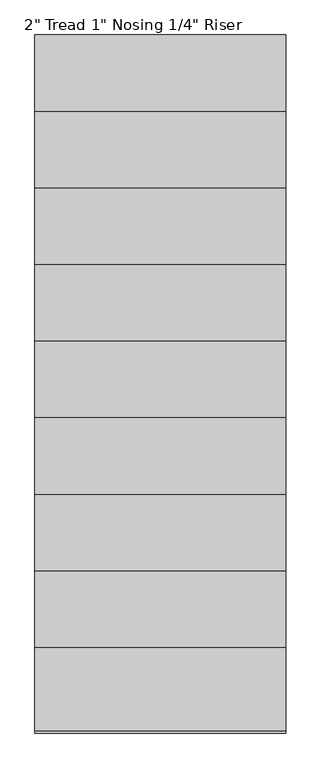
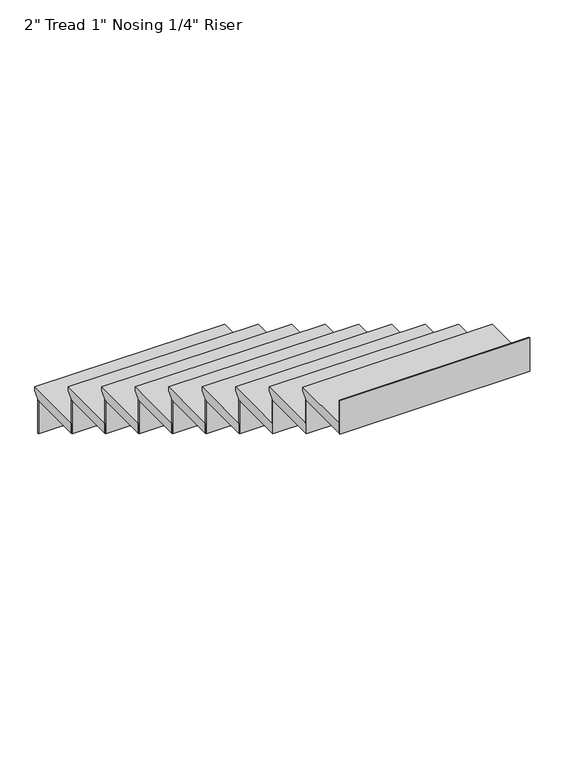
"""IFC4 building model written with IfcOpenShell, lengths in millimetres: stair flight geometry."""

from ifc_helpers import new_model, si_unit, frame, origin, place, context, project, spatial, polyline, outline, extrude, source, transform, mapped, element, save


def stair_flight_611140c6(model_context):
    return source(origin(), model_context, "Body", "SweptSolid", [
        extrude(outline(polyline([(-1599.5249317, 2133.6), (-1294.7249317, 2133.6), (-1294.7249317, 2114.55), (-1320.1249317, 2089.15), (-1320.1249317, 2082.8), (-1599.5249317, 2082.8), (-1599.5249317, 2133.6)])), frame((-7372.0431792, 0.0, 0.0), z_axis=(1.0, 0.0, 0.0), x_axis=(0.0, 1.0, 0.0)), (0.0, 0.0, 1.0), 914.4),
        extrude(outline(polyline([(-7372.0431792, -1326.4749317), (-7372.0431792, -1320.1249317), (-6457.6431792, -1320.1249317), (-6457.6431792, -1326.4749317), (-7372.0431792, -1326.4749317)])), frame((0.0, 0.0, 1913.4666667), z_axis=(0.0, 0.0, 1.0), x_axis=(1.0, 0.0, 0.0)), (0.0, 0.0, 1.0), 169.3333333),
        extrude(outline(polyline([(-7372.0431792, -1605.8749317), (-7372.0431792, -1599.5249317), (-6457.6431792, -1599.5249317), (-6457.6431792, -1605.8749317), (-7372.0431792, -1605.8749317)])), frame((0.0, 0.0, 2082.8), z_axis=(0.0, 0.0, 1.0), x_axis=(1.0, 0.0, 0.0)), (0.0, 0.0, 1.0), 169.3333333),
        extrude(outline(polyline([(-1878.9249317, 2302.9333333), (-1574.1249317, 2302.9333333), (-1574.1249317, 2283.8833333), (-1599.5249317, 2258.4833333), (-1599.5249317, 2252.1333333), (-1878.9249317, 2252.1333333), (-1878.9249317, 2302.9333333)])), frame((-7372.0431792, 0.0, 0.0), z_axis=(1.0, 0.0, 0.0), x_axis=(0.0, 1.0, 0.0)), (0.0, 0.0, 1.0), 914.4),
        extrude(outline(polyline([(-7372.0431792, -1885.2749317), (-7372.0431792, -1878.9249317), (-6457.6431792, -1878.9249317), (-6457.6431792, -1885.2749317), (-7372.0431792, -1885.2749317)])), frame((0.0, 0.0, 2252.1333333), z_axis=(0.0, 0.0, 1.0), x_axis=(1.0, 0.0, 0.0)), (0.0, 0.0, 1.0), 169.3333333),
        extrude(outline(polyline([(-2158.3249317, 2472.2666667), (-1853.5249317, 2472.2666667), (-1853.5249317, 2453.2166667), (-1878.9249317, 2427.8166667), (-1878.9249317, 2421.4666667), (-2158.3249317, 2421.4666667), (-2158.3249317, 2472.2666667)])), frame((-7372.0431792, 0.0, 0.0), z_axis=(1.0, 0.0, 0.0), x_axis=(0.0, 1.0, 0.0)), (0.0, 0.0, 1.0), 914.4),
        extrude(outline(polyline([(-7372.0431792, -2164.6749317), (-7372.0431792, -2158.3249317), (-6457.6431792, -2158.3249317), (-6457.6431792, -2164.6749317), (-7372.0431792, -2164.6749317)])), frame((0.0, 0.0, 2421.4666667), z_axis=(0.0, 0.0, 1.0), x_axis=(1.0, 0.0, 0.0)), (0.0, 0.0, 1.0), 169.3333333),
        extrude(outline(polyline([(-2437.7249317, 2641.6), (-2132.9249317, 2641.6), (-2132.9249317, 2622.55), (-2158.3249317, 2597.15), (-2158.3249317, 2590.8), (-2437.7249317, 2590.8), (-2437.7249317, 2641.6)])), frame((-7372.0431792, 0.0, 0.0), z_axis=(1.0, 0.0, 0.0), x_axis=(0.0, 1.0, 0.0)), (0.0, 0.0, 1.0), 914.4),
        extrude(outline(polyline([(-7372.0431792, -2444.0749317), (-7372.0431792, -2437.7249317), (-6457.6431792, -2437.7249317), (-6457.6431792, -2444.0749317), (-7372.0431792, -2444.0749317)])), frame((0.0, 0.0, 2590.8), z_axis=(0.0, 0.0, 1.0), x_axis=(1.0, 0.0, 0.0)), (0.0, 0.0, 1.0), 169.3333333),
        extrude(outline(polyline([(-2717.1249317, 2810.9333333), (-2412.3249317, 2810.9333333), (-2412.3249317, 2791.8833333), (-2437.7249317, 2766.4833333), (-2437.7249317, 2760.1333333), (-2717.1249317, 2760.1333333), (-2717.1249317, 2810.9333333)])), frame((-7372.0431792, 0.0, 0.0), z_axis=(1.0, 0.0, 0.0), x_axis=(0.0, 1.0, 0.0)), (0.0, 0.0, 1.0), 914.4),
        extrude(outline(polyline([(-7372.0431792, -2723.4749317), (-7372.0431792, -2717.1249317), (-6457.6431792, -2717.1249317), (-6457.6431792, -2723.4749317), (-7372.0431792, -2723.4749317)])), frame((0.0, 0.0, 2760.1333333), z_axis=(0.0, 0.0, 1.0), x_axis=(1.0, 0.0, 0.0)), (0.0, 0.0, 1.0), 169.3333333),
        extrude(outline(polyline([(-2996.5249317, 2980.2666667), (-2691.7249317, 2980.2666667), (-2691.7249317, 2961.2166667), (-2717.1249317, 2935.8166667), (-2717.1249317, 2929.4666667), (-2996.5249317, 2929.4666667), (-2996.5249317, 2980.2666667)])), frame((-7372.0431792, 0.0, 0.0), z_axis=(1.0, 0.0, 0.0), x_axis=(0.0, 1.0, 0.0)), (0.0, 0.0, 1.0), 914.4),
        extrude(outline(polyline([(-7372.0431792, -3002.8749317), (-7372.0431792, -2996.5249317), (-6457.6431792, -2996.5249317), (-6457.6431792, -3002.8749317), (-7372.0431792, -3002.8749317)])), frame((0.0, 0.0, 2929.4666667), z_axis=(0.0, 0.0, 1.0), x_axis=(1.0, 0.0, 0.0)), (0.0, 0.0, 1.0), 169.3333333),
        extrude(outline(polyline([(-3275.9249317, 3149.6), (-2971.1249317, 3149.6), (-2971.1249317, 3130.55), (-2996.5249317, 3105.15), (-2996.5249317, 3098.8), (-3275.9249317, 3098.8), (-3275.9249317, 3149.6)])), frame((-7372.0431792, 0.0, 0.0), z_axis=(1.0, 0.0, 0.0), x_axis=(0.0, 1.0, 0.0)), (0.0, 0.0, 1.0), 914.4),
        extrude(outline(polyline([(-7372.0431792, -3282.2749317), (-7372.0431792, -3275.9249317), (-6457.6431792, -3275.9249317), (-6457.6431792, -3282.2749317), (-7372.0431792, -3282.2749317)])), frame((0.0, 0.0, 3098.8), z_axis=(0.0, 0.0, 1.0), x_axis=(1.0, 0.0, 0.0)), (0.0, 0.0, 1.0), 169.3333333),
        extrude(outline(polyline([(-3555.3249317, 3318.9333333), (-3250.5249317, 3318.9333333), (-3250.5249317, 3299.8833333), (-3275.9249317, 3274.4833333), (-3275.9249317, 3268.1333333), (-3555.3249317, 3268.1333333), (-3555.3249317, 3318.9333333)])), frame((-7372.0431792, 0.0, 0.0), z_axis=(1.0, 0.0, 0.0), x_axis=(0.0, 1.0, 0.0)), (0.0, 0.0, 1.0), 914.4),
        extrude(outline(polyline([(-7372.0431792, -3561.6749317), (-7372.0431792, -3555.3249317), (-6457.6431792, -3555.3249317), (-6457.6431792, -3561.6749317), (-7372.0431792, -3561.6749317)])), frame((0.0, 0.0, 3268.1333333), z_axis=(0.0, 0.0, 1.0), x_axis=(1.0, 0.0, 0.0)), (0.0, 0.0, 1.0), 169.3333333),
        extrude(outline(polyline([(-7372.0431792, -3841.0749317), (-7372.0431792, -3834.7249317), (-6457.6431792, -3834.7249317), (-6457.6431792, -3841.0749317), (-7372.0431792, -3841.0749317)])), frame((0.0, 0.0, 3437.4666667), z_axis=(0.0, 0.0, 1.0), x_axis=(1.0, 0.0, 0.0)), (0.0, 0.0, 1.0), 169.3333333),
        extrude(outline(polyline([(-3834.7249317, 3488.2666667), (-3529.9249317, 3488.2666667), (-3529.9249317, 3469.2166667), (-3555.3249317, 3443.8166667), (-3555.3249317, 3437.4666667), (-3834.7249317, 3437.4666667), (-3834.7249317, 3488.2666667)])), frame((-7372.0431792, 0.0, 0.0), z_axis=(1.0, 0.0, 0.0), x_axis=(0.0, 1.0, 0.0)), (0.0, 0.0, 1.0), 914.4),
    ])


if __name__ == "__main__":
    model = new_model("IFC4")
    model_context = context("Model", 3, world=origin())
    ifc_project = project(units=[si_unit("LENGTHUNIT", "METRE", prefix="MILLI")], contexts=[model_context])
    site = spatial("IfcSite", under=ifc_project)
    building = spatial("IfcBuilding", under=site)
    placement = place(None, origin())
    stair_flight_shape = stair_flight_611140c6(model_context)
    element("IfcStairFlight", 1, ObjectType="2\" Tread 1\" Nosing 1/4\" Riser", at=placement, inside=building, context=model_context, shape_type="MappedRepresentation", body=[
        mapped(stair_flight_shape, transform((0.0, 0.0, 0.0), x_axis=(1.0, 0.0, 0.0), y_axis=(0.0, 1.0, 0.0), z_axis=(0.0, 0.0, 1.0))),
    ])
    save(model, "model.ifc")
